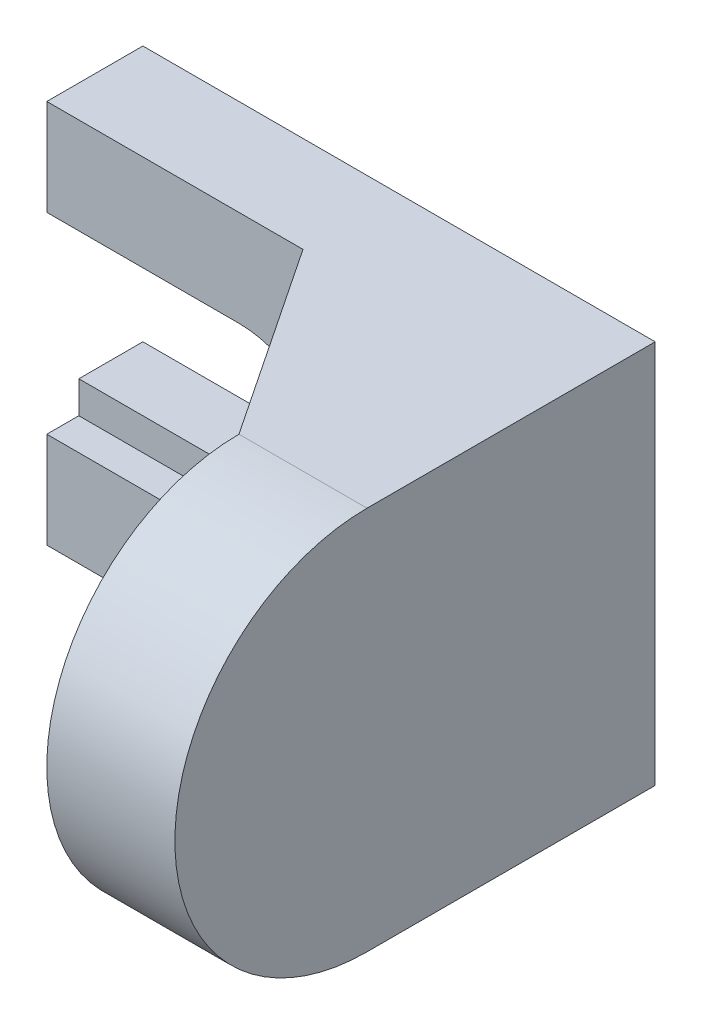
ISO-10303-21;
HEADER;
FILE_DESCRIPTION(('STEP AP214'),'2;1');
FILE_NAME('part.step','',(''),(''),'','','');
FILE_SCHEMA(('AUTOMOTIVE_DESIGN { 1 0 10303 214 1 1 1 1 }'));
ENDSEC;
DATA;
#1=APPLICATION_CONTEXT('core data for automotive mechanical design processes');
#2=APPLICATION_PROTOCOL_DEFINITION('international standard','automotive_design',2000,#1);
#3=PRODUCT_CONTEXT('',#1,'mechanical');
#4=PRODUCT('Part','Part','',(#3));
#5=PRODUCT_RELATED_PRODUCT_CATEGORY('part','',(#4));
#6=PRODUCT_DEFINITION_FORMATION('','',#4);
#7=PRODUCT_DEFINITION_CONTEXT('part definition',#1,'design');
#8=PRODUCT_DEFINITION('design','',#6,#7);
#9=PRODUCT_DEFINITION_SHAPE('','',#8);
#10=(LENGTH_UNIT() NAMED_UNIT(*) SI_UNIT(.MILLI.,.METRE.));
#11=(NAMED_UNIT(*) PLANE_ANGLE_UNIT() SI_UNIT($,.RADIAN.));
#12=(NAMED_UNIT(*) SI_UNIT($,.STERADIAN.) SOLID_ANGLE_UNIT());
#13=UNCERTAINTY_MEASURE_WITH_UNIT(LENGTH_MEASURE(1.E-05),#10,'distance_accuracy_value','');
#14=(GEOMETRIC_REPRESENTATION_CONTEXT(3) GLOBAL_UNCERTAINTY_ASSIGNED_CONTEXT((#13)) GLOBAL_UNIT_ASSIGNED_CONTEXT((#10,
#11,#12)) REPRESENTATION_CONTEXT('',''));
#15=CARTESIAN_POINT('',(0.,0.,0.));
#16=DIRECTION('',(0.,0.,1.));
#17=DIRECTION('',(1.,0.,0.));
#18=AXIS2_PLACEMENT_3D('',#15,#16,#17);
#19=CARTESIAN_POINT('',(0.,60.,15.));
#20=DIRECTION('',(1.,0.,0.));
#21=DIRECTION('',(0.,0.,-1.));
#22=AXIS2_PLACEMENT_3D('',#19,#20,#21);
#23=PLANE('',#22);
#24=DIRECTION('',(0.,-1.,0.));
#25=VECTOR('',#24,1.);
#26=CARTESIAN_POINT('',(0.,60.,0.));
#27=LINE('',#26,#25);
#28=CARTESIAN_POINT('',(0.,60.,0.));
#29=VERTEX_POINT('',#28);
#30=CARTESIAN_POINT('',(0.,40.,0.));
#31=VERTEX_POINT('',#30);
#32=EDGE_CURVE('E300',#29,#31,#27,.T.);
#33=ORIENTED_EDGE('',*,*,#32,.T.);
#34=DIRECTION('',(0.,0.,1.));
#35=VECTOR('',#34,1.);
#36=CARTESIAN_POINT('',(0.,40.,0.));
#37=LINE('',#36,#35);
#38=CARTESIAN_POINT('',(0.,40.,10.));
#39=VERTEX_POINT('',#38);
#40=EDGE_CURVE('E226',#31,#39,#37,.T.);
#41=ORIENTED_EDGE('',*,*,#40,.T.);
#42=DIRECTION('',(0.,-1.,0.));
#43=VECTOR('',#42,1.);
#44=CARTESIAN_POINT('',(0.,45.,10.));
#45=LINE('',#44,#43);
#46=CARTESIAN_POINT('',(0.,45.,10.));
#47=VERTEX_POINT('',#46);
#48=EDGE_CURVE('E239',#47,#39,#45,.T.);
#49=ORIENTED_EDGE('',*,*,#48,.F.);
#50=DIRECTION('',(0.,0.,1.));
#51=VECTOR('',#50,1.);
#52=CARTESIAN_POINT('',(0.,45.,10.));
#53=LINE('',#52,#51);
#54=CARTESIAN_POINT('',(0.,45.,15.));
#55=VERTEX_POINT('',#54);
#56=EDGE_CURVE('E250',#47,#55,#53,.T.);
#57=ORIENTED_EDGE('',*,*,#56,.T.);
#58=DIRECTION('',(0.,-1.,0.));
#59=VECTOR('',#58,1.);
#60=CARTESIAN_POINT('',(0.,60.,15.));
#61=LINE('',#60,#59);
#62=CARTESIAN_POINT('',(0.,60.,15.));
#63=VERTEX_POINT('',#62);
#64=EDGE_CURVE('E289',#63,#55,#61,.T.);
#65=ORIENTED_EDGE('',*,*,#64,.F.);
#66=DIRECTION('',(0.,0.,-1.));
#67=VECTOR('',#66,1.);
#68=CARTESIAN_POINT('',(0.,60.,15.));
#69=LINE('',#68,#67);
#70=EDGE_CURVE('E298',#63,#29,#69,.T.);
#71=ORIENTED_EDGE('',*,*,#70,.T.);
#72=EDGE_LOOP('',(#33,#41,#49,#57,#65,#71));
#73=FACE_BOUND('',#72,.T.);
#74=ADVANCED_FACE('F44',(#73),#23,.F.);
#75=CARTESIAN_POINT('',(0.,0.,15.));
#76=DIRECTION('',(0.,0.,1.));
#77=DIRECTION('',(1.,0.,0.));
#78=AXIS2_PLACEMENT_3D('',#75,#76,#77);
#79=PLANE('',#78);
#80=DIRECTION('',(0.,1.,0.));
#81=VECTOR('',#80,1.);
#82=CARTESIAN_POINT('',(40.,50.,15.));
#83=LINE('',#82,#81);
#84=CARTESIAN_POINT('',(40.,50.,15.));
#85=VERTEX_POINT('',#84);
#86=CARTESIAN_POINT('',(40.,60.,15.));
#87=VERTEX_POINT('',#86);
#88=EDGE_CURVE('E183',#85,#87,#83,.T.);
#89=ORIENTED_EDGE('',*,*,#88,.T.);
#90=DIRECTION('',(-1.,0.,0.));
#91=VECTOR('',#90,1.);
#92=CARTESIAN_POINT('',(80.,60.,15.));
#93=LINE('',#92,#91);
#94=EDGE_CURVE('E295',#87,#63,#93,.T.);
#95=ORIENTED_EDGE('',*,*,#94,.T.);
#96=ORIENTED_EDGE('',*,*,#64,.T.);
#97=DIRECTION('',(-1.,0.,0.));
#98=VECTOR('',#97,1.);
#99=CARTESIAN_POINT('',(0.,45.,15.));
#100=LINE('',#99,#98);
#101=CARTESIAN_POINT('',(30.,45.,15.));
#102=VERTEX_POINT('',#101);
#103=EDGE_CURVE('E233',#102,#55,#100,.T.);
#104=ORIENTED_EDGE('',*,*,#103,.F.);
#105=CARTESIAN_POINT('',(30.,30.,15.));
#106=DIRECTION('',(0.,0.,1.));
#107=DIRECTION('',(1.,0.,0.));
#108=AXIS2_PLACEMENT_3D('',#105,#106,#107);
#109=CIRCLE('',#108,15.);
#110=CARTESIAN_POINT('',(30.,15.,15.));
#111=VERTEX_POINT('',#110);
#112=EDGE_CURVE('E237',#111,#102,#109,.T.);
#113=ORIENTED_EDGE('',*,*,#112,.F.);
#114=DIRECTION('',(1.,0.,0.));
#115=VECTOR('',#114,1.);
#116=CARTESIAN_POINT('',(30.,15.,15.));
#117=LINE('',#116,#115);
#118=CARTESIAN_POINT('',(0.,15.,15.));
#119=VERTEX_POINT('',#118);
#120=EDGE_CURVE('E248',#119,#111,#117,.T.);
#121=ORIENTED_EDGE('',*,*,#120,.F.);
#122=CARTESIAN_POINT('',(0.,0.,15.));
#123=VERTEX_POINT('',#122);
#124=EDGE_CURVE('E293',#119,#123,#61,.T.);
#125=ORIENTED_EDGE('',*,*,#124,.T.);
#126=DIRECTION('',(1.,0.,0.));
#127=VECTOR('',#126,1.);
#128=CARTESIAN_POINT('',(0.,0.,15.));
#129=LINE('',#128,#127);
#130=CARTESIAN_POINT('',(40.,0.,15.));
#131=VERTEX_POINT('',#130);
#132=EDGE_CURVE('E288',#123,#131,#129,.T.);
#133=ORIENTED_EDGE('',*,*,#132,.T.);
#134=DIRECTION('',(0.,-1.,0.));
#135=VECTOR('',#134,1.);
#136=CARTESIAN_POINT('',(40.,10.,15.));
#137=LINE('',#136,#135);
#138=CARTESIAN_POINT('',(40.,10.,15.));
#139=VERTEX_POINT('',#138);
#140=EDGE_CURVE('E209',#139,#131,#137,.T.);
#141=ORIENTED_EDGE('',*,*,#140,.F.);
#142=DIRECTION('',(1.,0.,0.));
#143=VECTOR('',#142,1.);
#144=CARTESIAN_POINT('',(60.,10.,15.));
#145=LINE('',#144,#143);
#146=CARTESIAN_POINT('',(60.,10.,15.));
#147=VERTEX_POINT('',#146);
#148=EDGE_CURVE('E205',#139,#147,#145,.T.);
#149=ORIENTED_EDGE('',*,*,#148,.T.);
#150=DIRECTION('',(0.,1.,0.));
#151=VECTOR('',#150,1.);
#152=CARTESIAN_POINT('',(60.,0.,15.));
#153=LINE('',#152,#151);
#154=CARTESIAN_POINT('',(60.,50.,15.));
#155=VERTEX_POINT('',#154);
#156=EDGE_CURVE('E273',#147,#155,#153,.T.);
#157=ORIENTED_EDGE('',*,*,#156,.T.);
#158=DIRECTION('',(-1.,0.,0.));
#159=VECTOR('',#158,1.);
#160=CARTESIAN_POINT('',(40.,50.,15.));
#161=LINE('',#160,#159);
#162=EDGE_CURVE('E175',#155,#85,#161,.T.);
#163=ORIENTED_EDGE('',*,*,#162,.T.);
#164=EDGE_LOOP('',(#89,#95,#96,#104,#113,#121,#125,#133,#141,#149,#157,#163));
#165=FACE_BOUND('',#164,.T.);
#166=ADVANCED_FACE('F334',(#165),#79,.T.);
#167=CARTESIAN_POINT('',(0.,20.,10.));
#168=VERTEX_POINT('',#167);
#169=CARTESIAN_POINT('',(0.,15.,10.));
#170=VERTEX_POINT('',#169);
#171=EDGE_CURVE('E238',#168,#170,#45,.T.);
#172=ORIENTED_EDGE('',*,*,#171,.F.);
#173=DIRECTION('',(0.,0.,1.));
#174=VECTOR('',#173,1.);
#175=CARTESIAN_POINT('',(0.,20.,0.));
#176=LINE('',#175,#174);
#177=CARTESIAN_POINT('',(0.,20.,0.));
#178=VERTEX_POINT('',#177);
#179=EDGE_CURVE('E58',#178,#168,#176,.T.);
#180=ORIENTED_EDGE('',*,*,#179,.F.);
#181=CARTESIAN_POINT('',(0.,0.,0.));
#182=VERTEX_POINT('',#181);
#183=EDGE_CURVE('E282',#178,#182,#27,.T.);
#184=ORIENTED_EDGE('',*,*,#183,.T.);
#185=DIRECTION('',(0.,0.,-1.));
#186=VECTOR('',#185,1.);
#187=CARTESIAN_POINT('',(0.,0.,15.));
#188=LINE('',#187,#186);
#189=EDGE_CURVE('E11',#123,#182,#188,.T.);
#190=ORIENTED_EDGE('',*,*,#189,.F.);
#191=ORIENTED_EDGE('',*,*,#124,.F.);
#192=DIRECTION('',(0.,0.,1.));
#193=VECTOR('',#192,1.);
#194=CARTESIAN_POINT('',(0.,15.,10.));
#195=LINE('',#194,#193);
#196=EDGE_CURVE('E256',#170,#119,#195,.T.);
#197=ORIENTED_EDGE('',*,*,#196,.F.);
#198=EDGE_LOOP('',(#172,#180,#184,#190,#191,#197));
#199=FACE_BOUND('',#198,.T.);
#200=ADVANCED_FACE('F50',(#199),#23,.F.);
#201=CARTESIAN_POINT('',(0.,0.,15.));
#202=DIRECTION('',(0.,1.,0.));
#203=DIRECTION('',(0.,0.,1.));
#204=AXIS2_PLACEMENT_3D('',#201,#202,#203);
#205=PLANE('',#204);
#206=DIRECTION('',(1.,0.,0.));
#207=VECTOR('',#206,1.);
#208=CARTESIAN_POINT('',(0.,0.,0.));
#209=LINE('',#208,#207);
#210=CARTESIAN_POINT('',(80.,0.,0.));
#211=VERTEX_POINT('',#210);
#212=EDGE_CURVE('E297',#182,#211,#209,.T.);
#213=ORIENTED_EDGE('',*,*,#212,.T.);
#214=DIRECTION('',(0.,0.,-1.));
#215=VECTOR('',#214,1.);
#216=CARTESIAN_POINT('',(80.,0.,15.));
#217=LINE('',#216,#215);
#218=CARTESIAN_POINT('',(80.,0.,45.));
#219=VERTEX_POINT('',#218);
#220=EDGE_CURVE('E52',#219,#211,#217,.T.);
#221=ORIENTED_EDGE('',*,*,#220,.F.);
#222=DIRECTION('',(1.,0.,0.));
#223=VECTOR('',#222,1.);
#224=CARTESIAN_POINT('',(60.,0.,45.));
#225=LINE('',#224,#223);
#226=CARTESIAN_POINT('',(60.,0.,45.));
#227=VERTEX_POINT('',#226);
#228=EDGE_CURVE('E283',#227,#219,#225,.T.);
#229=ORIENTED_EDGE('',*,*,#228,.F.);
#230=DIRECTION('',(-0.554700196225229,0.,-0.832050294337844));
#231=VECTOR('',#230,1.);
#232=CARTESIAN_POINT('',(60.,0.,45.));
#233=LINE('',#232,#231);
#234=EDGE_CURVE('E194',#227,#131,#233,.T.);
#235=ORIENTED_EDGE('',*,*,#234,.T.);
#236=ORIENTED_EDGE('',*,*,#132,.F.);
#237=ORIENTED_EDGE('',*,*,#189,.T.);
#238=EDGE_LOOP('',(#213,#221,#229,#235,#236,#237));
#239=FACE_BOUND('',#238,.T.);
#240=ADVANCED_FACE('F337',(#239),#205,.F.);
#241=CARTESIAN_POINT('',(80.,0.,15.));
#242=DIRECTION('',(-1.,0.,0.));
#243=DIRECTION('',(0.,0.,1.));
#244=AXIS2_PLACEMENT_3D('',#241,#242,#243);
#245=PLANE('',#244);
#246=DIRECTION('',(0.,1.,0.));
#247=VECTOR('',#246,1.);
#248=CARTESIAN_POINT('',(80.,0.,0.));
#249=LINE('',#248,#247);
#250=CARTESIAN_POINT('',(80.,60.,0.));
#251=VERTEX_POINT('',#250);
#252=EDGE_CURVE('E305',#211,#251,#249,.T.);
#253=ORIENTED_EDGE('',*,*,#252,.T.);
#254=DIRECTION('',(0.,0.,-1.));
#255=VECTOR('',#254,1.);
#256=CARTESIAN_POINT('',(80.,60.,15.));
#257=LINE('',#256,#255);
#258=CARTESIAN_POINT('',(80.,60.,45.));
#259=VERTEX_POINT('',#258);
#260=EDGE_CURVE('E308',#259,#251,#257,.T.);
#261=ORIENTED_EDGE('',*,*,#260,.F.);
#262=CARTESIAN_POINT('',(80.,30.,45.));
#263=DIRECTION('',(1.,0.,0.));
#264=DIRECTION('',(0.,0.,-1.));
#265=AXIS2_PLACEMENT_3D('',#262,#263,#264);
#266=CIRCLE('',#265,30.);
#267=EDGE_CURVE('E275',#259,#219,#266,.T.);
#268=ORIENTED_EDGE('',*,*,#267,.T.);
#269=ORIENTED_EDGE('',*,*,#220,.T.);
#270=EDGE_LOOP('',(#253,#261,#268,#269));
#271=FACE_BOUND('',#270,.T.);
#272=ADVANCED_FACE('F312',(#271),#245,.F.);
#273=CARTESIAN_POINT('',(80.,60.,15.));
#274=DIRECTION('',(0.,-1.,0.));
#275=DIRECTION('',(0.,0.,-1.));
#276=AXIS2_PLACEMENT_3D('',#273,#274,#275);
#277=PLANE('',#276);
#278=ORIENTED_EDGE('',*,*,#94,.F.);
#279=DIRECTION('',(0.554700196225229,0.,0.832050294337844));
#280=VECTOR('',#279,1.);
#281=CARTESIAN_POINT('',(60.,60.,45.));
#282=LINE('',#281,#280);
#283=CARTESIAN_POINT('',(60.,60.,45.));
#284=VERTEX_POINT('',#283);
#285=EDGE_CURVE('E184',#87,#284,#282,.T.);
#286=ORIENTED_EDGE('',*,*,#285,.T.);
#287=DIRECTION('',(1.,0.,0.));
#288=VECTOR('',#287,1.);
#289=CARTESIAN_POINT('',(60.,60.,45.));
#290=LINE('',#289,#288);
#291=EDGE_CURVE('E279',#284,#259,#290,.T.);
#292=ORIENTED_EDGE('',*,*,#291,.T.);
#293=ORIENTED_EDGE('',*,*,#260,.T.);
#294=DIRECTION('',(-1.,0.,0.));
#295=VECTOR('',#294,1.);
#296=CARTESIAN_POINT('',(80.,60.,0.));
#297=LINE('',#296,#295);
#298=EDGE_CURVE('E302',#251,#29,#297,.T.);
#299=ORIENTED_EDGE('',*,*,#298,.T.);
#300=ORIENTED_EDGE('',*,*,#70,.F.);
#301=EDGE_LOOP('',(#278,#286,#292,#293,#299,#300));
#302=FACE_BOUND('',#301,.T.);
#303=ADVANCED_FACE('F328',(#302),#277,.F.);
#304=CARTESIAN_POINT('',(0.,0.,0.));
#305=DIRECTION('',(0.,0.,1.));
#306=DIRECTION('',(1.,0.,0.));
#307=AXIS2_PLACEMENT_3D('',#304,#305,#306);
#308=PLANE('',#307);
#309=CARTESIAN_POINT('',(29.9999999999999,30.,0.));
#310=DIRECTION('',(0.,0.,1.));
#311=DIRECTION('',(1.,0.,0.));
#312=AXIS2_PLACEMENT_3D('',#309,#310,#311);
#313=CIRCLE('',#312,10.);
#314=CARTESIAN_POINT('',(29.9999999999999,20.,0.));
#315=VERTEX_POINT('',#314);
#316=CARTESIAN_POINT('',(29.9999999999999,40.,0.));
#317=VERTEX_POINT('',#316);
#318=EDGE_CURVE('E218',#315,#317,#313,.T.);
#319=ORIENTED_EDGE('',*,*,#318,.T.);
#320=DIRECTION('',(-1.,0.,0.));
#321=VECTOR('',#320,1.);
#322=CARTESIAN_POINT('',(0.,40.,0.));
#323=LINE('',#322,#321);
#324=EDGE_CURVE('E219',#317,#31,#323,.T.);
#325=ORIENTED_EDGE('',*,*,#324,.T.);
#326=ORIENTED_EDGE('',*,*,#32,.F.);
#327=ORIENTED_EDGE('',*,*,#298,.F.);
#328=ORIENTED_EDGE('',*,*,#252,.F.);
#329=ORIENTED_EDGE('',*,*,#212,.F.);
#330=ORIENTED_EDGE('',*,*,#183,.F.);
#331=DIRECTION('',(1.,0.,0.));
#332=VECTOR('',#331,1.);
#333=CARTESIAN_POINT('',(0.,20.,0.));
#334=LINE('',#333,#332);
#335=EDGE_CURVE('E214',#178,#315,#334,.T.);
#336=ORIENTED_EDGE('',*,*,#335,.T.);
#337=EDGE_LOOP('',(#319,#325,#326,#327,#328,#329,#330,#336));
#338=FACE_BOUND('',#337,.T.);
#339=ADVANCED_FACE('F318',(#338),#308,.F.);
#340=CARTESIAN_POINT('',(60.,30.,45.));
#341=DIRECTION('',(1.,0.,0.));
#342=DIRECTION('',(0.,0.,-1.));
#343=AXIS2_PLACEMENT_3D('',#340,#341,#342);
#344=CYLINDRICAL_SURFACE('',#343,30.);
#345=ORIENTED_EDGE('',*,*,#267,.F.);
#346=ORIENTED_EDGE('',*,*,#291,.F.);
#347=CARTESIAN_POINT('',(60.,30.,45.));
#348=DIRECTION('',(1.,0.,0.));
#349=DIRECTION('',(0.,0.,-1.));
#350=AXIS2_PLACEMENT_3D('',#347,#348,#349);
#351=CIRCLE('',#350,30.);
#352=EDGE_CURVE('E192',#284,#227,#351,.T.);
#353=ORIENTED_EDGE('',*,*,#352,.T.);
#354=ORIENTED_EDGE('',*,*,#228,.T.);
#355=EDGE_LOOP('',(#345,#346,#353,#354));
#356=FACE_BOUND('',#355,.T.);
#357=ADVANCED_FACE('F333',(#356),#344,.T.);
#358=CARTESIAN_POINT('',(60.,30.,45.));
#359=DIRECTION('',(1.,0.,0.));
#360=DIRECTION('',(0.,0.,-1.));
#361=AXIS2_PLACEMENT_3D('',#358,#359,#360);
#362=PLANE('',#361);
#363=CARTESIAN_POINT('',(60.,30.,45.));
#364=DIRECTION('',(-1.,0.,0.));
#365=DIRECTION('',(0.,0.,1.));
#366=AXIS2_PLACEMENT_3D('',#363,#364,#365);
#367=CIRCLE('',#366,15.);
#368=CARTESIAN_POINT('',(60.,30.,60.));
#369=VERTEX_POINT('',#368);
#370=EDGE_CURVE('E267',#369,#369,#367,.T.);
#371=ORIENTED_EDGE('',*,*,#370,.F.);
#372=EDGE_LOOP('',(#371));
#373=FACE_BOUND('',#372,.T.);
#374=ORIENTED_EDGE('',*,*,#352,.F.);
#375=DIRECTION('',(0.,1.,0.));
#376=VECTOR('',#375,1.);
#377=CARTESIAN_POINT('',(60.,50.,45.));
#378=LINE('',#377,#376);
#379=CARTESIAN_POINT('',(60.,50.,45.));
#380=VERTEX_POINT('',#379);
#381=EDGE_CURVE('E181',#380,#284,#378,.T.);
#382=ORIENTED_EDGE('',*,*,#381,.F.);
#383=DIRECTION('',(0.,0.,-1.));
#384=VECTOR('',#383,1.);
#385=CARTESIAN_POINT('',(60.,50.,15.));
#386=LINE('',#385,#384);
#387=EDGE_CURVE('E170',#380,#155,#386,.T.);
#388=ORIENTED_EDGE('',*,*,#387,.T.);
#389=ORIENTED_EDGE('',*,*,#156,.F.);
#390=DIRECTION('',(0.,0.,1.));
#391=VECTOR('',#390,1.);
#392=CARTESIAN_POINT('',(60.,10.,45.));
#393=LINE('',#392,#391);
#394=CARTESIAN_POINT('',(60.,10.,45.));
#395=VERTEX_POINT('',#394);
#396=EDGE_CURVE('E196',#147,#395,#393,.T.);
#397=ORIENTED_EDGE('',*,*,#396,.T.);
#398=DIRECTION('',(0.,-1.,0.));
#399=VECTOR('',#398,1.);
#400=CARTESIAN_POINT('',(60.,10.,45.));
#401=LINE('',#400,#399);
#402=EDGE_CURVE('E207',#395,#227,#401,.T.);
#403=ORIENTED_EDGE('',*,*,#402,.T.);
#404=EDGE_LOOP('',(#374,#382,#388,#389,#397,#403));
#405=FACE_BOUND('',#404,.T.);
#406=ADVANCED_FACE('F189',(#373,#405),#362,.F.);
#407=CARTESIAN_POINT('',(65.,30.,45.));
#408=DIRECTION('',(-1.,0.,0.));
#409=DIRECTION('',(0.,0.,1.));
#410=AXIS2_PLACEMENT_3D('',#407,#408,#409);
#411=CYLINDRICAL_SURFACE('',#410,15.);
#412=CARTESIAN_POINT('',(65.,30.,45.));
#413=DIRECTION('',(-1.,0.,0.));
#414=DIRECTION('',(0.,0.,1.));
#415=AXIS2_PLACEMENT_3D('',#412,#413,#414);
#416=CIRCLE('',#415,15.);
#417=CARTESIAN_POINT('',(65.,30.,60.));
#418=VERTEX_POINT('',#417);
#419=EDGE_CURVE('E266',#418,#418,#416,.T.);
#420=ORIENTED_EDGE('',*,*,#419,.F.);
#421=EDGE_LOOP('',(#420));
#422=FACE_BOUND('',#421,.T.);
#423=ORIENTED_EDGE('',*,*,#370,.T.);
#424=EDGE_LOOP('',(#423));
#425=FACE_BOUND('',#424,.T.);
#426=ADVANCED_FACE('F400',(#422,#425),#411,.F.);
#427=CARTESIAN_POINT('',(65.,30.,45.));
#428=DIRECTION('',(-1.,0.,0.));
#429=DIRECTION('',(0.,0.,1.));
#430=AXIS2_PLACEMENT_3D('',#427,#428,#429);
#431=PLANE('',#430);
#432=CARTESIAN_POINT('',(65.,30.,45.));
#433=DIRECTION('',(-1.,0.,0.));
#434=DIRECTION('',(0.,0.,1.));
#435=AXIS2_PLACEMENT_3D('',#432,#433,#434);
#436=CIRCLE('',#435,10.);
#437=CARTESIAN_POINT('',(65.,30.,55.));
#438=VERTEX_POINT('',#437);
#439=EDGE_CURVE('E257',#438,#438,#436,.T.);
#440=ORIENTED_EDGE('',*,*,#439,.F.);
#441=EDGE_LOOP('',(#440));
#442=FACE_BOUND('',#441,.T.);
#443=ORIENTED_EDGE('',*,*,#419,.T.);
#444=EDGE_LOOP('',(#443));
#445=FACE_BOUND('',#444,.T.);
#446=ADVANCED_FACE('F405',(#442,#445),#431,.T.);
#447=CARTESIAN_POINT('',(70.,30.,45.));
#448=DIRECTION('',(-1.,0.,0.));
#449=DIRECTION('',(0.,0.,1.));
#450=AXIS2_PLACEMENT_3D('',#447,#448,#449);
#451=CYLINDRICAL_SURFACE('',#450,10.);
#452=CARTESIAN_POINT('',(70.,30.,45.));
#453=DIRECTION('',(-1.,0.,0.));
#454=DIRECTION('',(0.,0.,1.));
#455=AXIS2_PLACEMENT_3D('',#452,#453,#454);
#456=CIRCLE('',#455,10.);
#457=CARTESIAN_POINT('',(70.,30.,55.));
#458=VERTEX_POINT('',#457);
#459=EDGE_CURVE('E261',#458,#458,#456,.T.);
#460=ORIENTED_EDGE('',*,*,#459,.F.);
#461=EDGE_LOOP('',(#460));
#462=FACE_BOUND('',#461,.T.);
#463=ORIENTED_EDGE('',*,*,#439,.T.);
#464=EDGE_LOOP('',(#463));
#465=FACE_BOUND('',#464,.T.);
#466=ADVANCED_FACE('F375',(#462,#465),#451,.F.);
#467=CARTESIAN_POINT('',(70.,30.,45.));
#468=DIRECTION('',(-1.,0.,0.));
#469=DIRECTION('',(0.,0.,1.));
#470=AXIS2_PLACEMENT_3D('',#467,#468,#469);
#471=PLANE('',#470);
#472=ORIENTED_EDGE('',*,*,#459,.T.);
#473=EDGE_LOOP('',(#472));
#474=FACE_BOUND('',#473,.T.);
#475=ADVANCED_FACE('F362',(#474),#471,.T.);
#476=CARTESIAN_POINT('',(0.,45.,10.));
#477=DIRECTION('',(0.,1.,0.));
#478=DIRECTION('',(0.,0.,1.));
#479=AXIS2_PLACEMENT_3D('',#476,#477,#478);
#480=PLANE('',#479);
#481=ORIENTED_EDGE('',*,*,#103,.T.);
#482=ORIENTED_EDGE('',*,*,#56,.F.);
#483=DIRECTION('',(-1.,0.,0.));
#484=VECTOR('',#483,1.);
#485=CARTESIAN_POINT('',(0.,45.,10.));
#486=LINE('',#485,#484);
#487=CARTESIAN_POINT('',(30.,45.,10.));
#488=VERTEX_POINT('',#487);
#489=EDGE_CURVE('E66',#488,#47,#486,.T.);
#490=ORIENTED_EDGE('',*,*,#489,.F.);
#491=DIRECTION('',(0.,0.,1.));
#492=VECTOR('',#491,1.);
#493=CARTESIAN_POINT('',(30.,45.,10.));
#494=LINE('',#493,#492);
#495=EDGE_CURVE('E251',#488,#102,#494,.T.);
#496=ORIENTED_EDGE('',*,*,#495,.T.);
#497=EDGE_LOOP('',(#481,#482,#490,#496));
#498=FACE_BOUND('',#497,.T.);
#499=ADVANCED_FACE('F361',(#498),#480,.F.);
#500=CARTESIAN_POINT('',(30.,30.,10.));
#501=DIRECTION('',(0.,0.,1.));
#502=DIRECTION('',(1.,0.,0.));
#503=AXIS2_PLACEMENT_3D('',#500,#501,#502);
#504=CYLINDRICAL_SURFACE('',#503,15.);
#505=ORIENTED_EDGE('',*,*,#112,.T.);
#506=ORIENTED_EDGE('',*,*,#495,.F.);
#507=CARTESIAN_POINT('',(30.,30.,10.));
#508=DIRECTION('',(0.,0.,1.));
#509=DIRECTION('',(1.,0.,0.));
#510=AXIS2_PLACEMENT_3D('',#507,#508,#509);
#511=CIRCLE('',#510,15.);
#512=CARTESIAN_POINT('',(30.,15.,10.));
#513=VERTEX_POINT('',#512);
#514=EDGE_CURVE('E244',#513,#488,#511,.T.);
#515=ORIENTED_EDGE('',*,*,#514,.F.);
#516=DIRECTION('',(0.,0.,1.));
#517=VECTOR('',#516,1.);
#518=CARTESIAN_POINT('',(30.,15.,10.));
#519=LINE('',#518,#517);
#520=EDGE_CURVE('E260',#513,#111,#519,.T.);
#521=ORIENTED_EDGE('',*,*,#520,.T.);
#522=EDGE_LOOP('',(#505,#506,#515,#521));
#523=FACE_BOUND('',#522,.T.);
#524=ADVANCED_FACE('F363',(#523),#504,.F.);
#525=CARTESIAN_POINT('',(30.,15.,10.));
#526=DIRECTION('',(0.,-1.,0.));
#527=DIRECTION('',(0.,0.,-1.));
#528=AXIS2_PLACEMENT_3D('',#525,#526,#527);
#529=PLANE('',#528);
#530=ORIENTED_EDGE('',*,*,#120,.T.);
#531=ORIENTED_EDGE('',*,*,#520,.F.);
#532=DIRECTION('',(1.,0.,0.));
#533=VECTOR('',#532,1.);
#534=CARTESIAN_POINT('',(30.,15.,10.));
#535=LINE('',#534,#533);
#536=EDGE_CURVE('E245',#170,#513,#535,.T.);
#537=ORIENTED_EDGE('',*,*,#536,.F.);
#538=ORIENTED_EDGE('',*,*,#196,.T.);
#539=EDGE_LOOP('',(#530,#531,#537,#538));
#540=FACE_BOUND('',#539,.T.);
#541=ADVANCED_FACE('F360',(#540),#529,.F.);
#542=CARTESIAN_POINT('',(30.,30.,10.));
#543=DIRECTION('',(0.,0.,1.));
#544=DIRECTION('',(1.,0.,0.));
#545=AXIS2_PLACEMENT_3D('',#542,#543,#544);
#546=PLANE('',#545);
#547=DIRECTION('',(-1.,0.,0.));
#548=VECTOR('',#547,1.);
#549=CARTESIAN_POINT('',(0.,40.,10.));
#550=LINE('',#549,#548);
#551=CARTESIAN_POINT('',(29.9999999999999,40.,10.));
#552=VERTEX_POINT('',#551);
#553=EDGE_CURVE('E220',#552,#39,#550,.T.);
#554=ORIENTED_EDGE('',*,*,#553,.F.);
#555=CARTESIAN_POINT('',(29.9999999999999,30.,10.));
#556=DIRECTION('',(0.,0.,1.));
#557=DIRECTION('',(1.,0.,0.));
#558=AXIS2_PLACEMENT_3D('',#555,#556,#557);
#559=CIRCLE('',#558,10.);
#560=CARTESIAN_POINT('',(29.9999999999999,20.,10.));
#561=VERTEX_POINT('',#560);
#562=EDGE_CURVE('E221',#561,#552,#559,.T.);
#563=ORIENTED_EDGE('',*,*,#562,.F.);
#564=DIRECTION('',(1.,0.,0.));
#565=VECTOR('',#564,1.);
#566=CARTESIAN_POINT('',(0.,20.,10.));
#567=LINE('',#566,#565);
#568=EDGE_CURVE('E212',#168,#561,#567,.T.);
#569=ORIENTED_EDGE('',*,*,#568,.F.);
#570=ORIENTED_EDGE('',*,*,#171,.T.);
#571=ORIENTED_EDGE('',*,*,#536,.T.);
#572=ORIENTED_EDGE('',*,*,#514,.T.);
#573=ORIENTED_EDGE('',*,*,#489,.T.);
#574=ORIENTED_EDGE('',*,*,#48,.T.);
#575=EDGE_LOOP('',(#554,#563,#569,#570,#571,#572,#573,#574));
#576=FACE_BOUND('',#575,.T.);
#577=ADVANCED_FACE('F353',(#576),#546,.T.);
#578=CARTESIAN_POINT('',(0.,40.,0.));
#579=DIRECTION('',(0.,1.,0.));
#580=DIRECTION('',(0.,0.,1.));
#581=AXIS2_PLACEMENT_3D('',#578,#579,#580);
#582=PLANE('',#581);
#583=ORIENTED_EDGE('',*,*,#553,.T.);
#584=ORIENTED_EDGE('',*,*,#40,.F.);
#585=ORIENTED_EDGE('',*,*,#324,.F.);
#586=DIRECTION('',(0.,0.,1.));
#587=VECTOR('',#586,1.);
#588=CARTESIAN_POINT('',(29.9999999999999,40.,0.));
#589=LINE('',#588,#587);
#590=EDGE_CURVE('E235',#317,#552,#589,.T.);
#591=ORIENTED_EDGE('',*,*,#590,.T.);
#592=EDGE_LOOP('',(#583,#584,#585,#591));
#593=FACE_BOUND('',#592,.T.);
#594=ADVANCED_FACE('F351',(#593),#582,.F.);
#595=CARTESIAN_POINT('',(29.9999999999999,30.,0.));
#596=DIRECTION('',(0.,0.,1.));
#597=DIRECTION('',(1.,0.,0.));
#598=AXIS2_PLACEMENT_3D('',#595,#596,#597);
#599=CYLINDRICAL_SURFACE('',#598,10.);
#600=ORIENTED_EDGE('',*,*,#562,.T.);
#601=ORIENTED_EDGE('',*,*,#590,.F.);
#602=ORIENTED_EDGE('',*,*,#318,.F.);
#603=DIRECTION('',(0.,0.,1.));
#604=VECTOR('',#603,1.);
#605=CARTESIAN_POINT('',(29.9999999999999,20.,0.));
#606=LINE('',#605,#604);
#607=EDGE_CURVE('E234',#315,#561,#606,.T.);
#608=ORIENTED_EDGE('',*,*,#607,.T.);
#609=EDGE_LOOP('',(#600,#601,#602,#608));
#610=FACE_BOUND('',#609,.T.);
#611=ADVANCED_FACE('F349',(#610),#599,.F.);
#612=CARTESIAN_POINT('',(0.,20.,0.));
#613=DIRECTION('',(0.,-1.,0.));
#614=DIRECTION('',(0.,0.,-1.));
#615=AXIS2_PLACEMENT_3D('',#612,#613,#614);
#616=PLANE('',#615);
#617=ORIENTED_EDGE('',*,*,#568,.T.);
#618=ORIENTED_EDGE('',*,*,#607,.F.);
#619=ORIENTED_EDGE('',*,*,#335,.F.);
#620=ORIENTED_EDGE('',*,*,#179,.T.);
#621=EDGE_LOOP('',(#617,#618,#619,#620));
#622=FACE_BOUND('',#621,.T.);
#623=ADVANCED_FACE('F350',(#622),#616,.F.);
#624=CARTESIAN_POINT('',(60.,10.,45.));
#625=DIRECTION('',(-0.832050294337844,0.,0.554700196225229));
#626=DIRECTION('',(0.554700196225229,0.,0.832050294337844));
#627=AXIS2_PLACEMENT_3D('',#624,#625,#626);
#628=PLANE('',#627);
#629=ORIENTED_EDGE('',*,*,#234,.F.);
#630=ORIENTED_EDGE('',*,*,#402,.F.);
#631=DIRECTION('',(-0.554700196225229,0.,-0.832050294337844));
#632=VECTOR('',#631,1.);
#633=CARTESIAN_POINT('',(60.,10.,45.));
#634=LINE('',#633,#632);
#635=EDGE_CURVE('E202',#395,#139,#634,.T.);
#636=ORIENTED_EDGE('',*,*,#635,.T.);
#637=ORIENTED_EDGE('',*,*,#140,.T.);
#638=EDGE_LOOP('',(#629,#630,#636,#637));
#639=FACE_BOUND('',#638,.T.);
#640=ADVANCED_FACE('F478',(#639),#628,.T.);
#641=CARTESIAN_POINT('',(0.,10.,0.));
#642=DIRECTION('',(0.,1.,0.));
#643=DIRECTION('',(0.,0.,1.));
#644=AXIS2_PLACEMENT_3D('',#641,#642,#643);
#645=PLANE('',#644);
#646=ORIENTED_EDGE('',*,*,#396,.F.);
#647=ORIENTED_EDGE('',*,*,#148,.F.);
#648=ORIENTED_EDGE('',*,*,#635,.F.);
#649=EDGE_LOOP('',(#646,#647,#648));
#650=FACE_BOUND('',#649,.T.);
#651=ADVANCED_FACE('F488',(#650),#645,.T.);
#652=CARTESIAN_POINT('',(60.,50.,45.));
#653=DIRECTION('',(-0.832050294337844,0.,0.554700196225229));
#654=DIRECTION('',(0.554700196225229,0.,0.832050294337844));
#655=AXIS2_PLACEMENT_3D('',#652,#653,#654);
#656=PLANE('',#655);
#657=ORIENTED_EDGE('',*,*,#285,.F.);
#658=ORIENTED_EDGE('',*,*,#88,.F.);
#659=DIRECTION('',(0.554700196225229,0.,0.832050294337844));
#660=VECTOR('',#659,1.);
#661=CARTESIAN_POINT('',(60.,50.,45.));
#662=LINE('',#661,#660);
#663=EDGE_CURVE('E167',#85,#380,#662,.T.);
#664=ORIENTED_EDGE('',*,*,#663,.T.);
#665=ORIENTED_EDGE('',*,*,#381,.T.);
#666=EDGE_LOOP('',(#657,#658,#664,#665));
#667=FACE_BOUND('',#666,.T.);
#668=ADVANCED_FACE('F179',(#667),#656,.T.);
#669=CARTESIAN_POINT('',(0.,50.,0.));
#670=DIRECTION('',(0.,-1.,0.));
#671=DIRECTION('',(0.,0.,-1.));
#672=AXIS2_PLACEMENT_3D('',#669,#670,#671);
#673=PLANE('',#672);
#674=ORIENTED_EDGE('',*,*,#663,.F.);
#675=ORIENTED_EDGE('',*,*,#162,.F.);
#676=ORIENTED_EDGE('',*,*,#387,.F.);
#677=EDGE_LOOP('',(#674,#675,#676));
#678=FACE_BOUND('',#677,.T.);
#679=ADVANCED_FACE('F169',(#678),#673,.T.);
#680=CLOSED_SHELL('',(#74,#166,#200,#240,#272,#303,#339,#357,#406,#426,#446,#466,#475,#499,#524,
#541,#577,#594,#611,#623,#640,#651,#668,#679));
#681=MANIFOLD_SOLID_BREP('B2',#680);
#682=ADVANCED_BREP_SHAPE_REPRESENTATION('',(#18,#681),#14);
#683=SHAPE_DEFINITION_REPRESENTATION(#9,#682);
ENDSEC;
END-ISO-10303-21;
